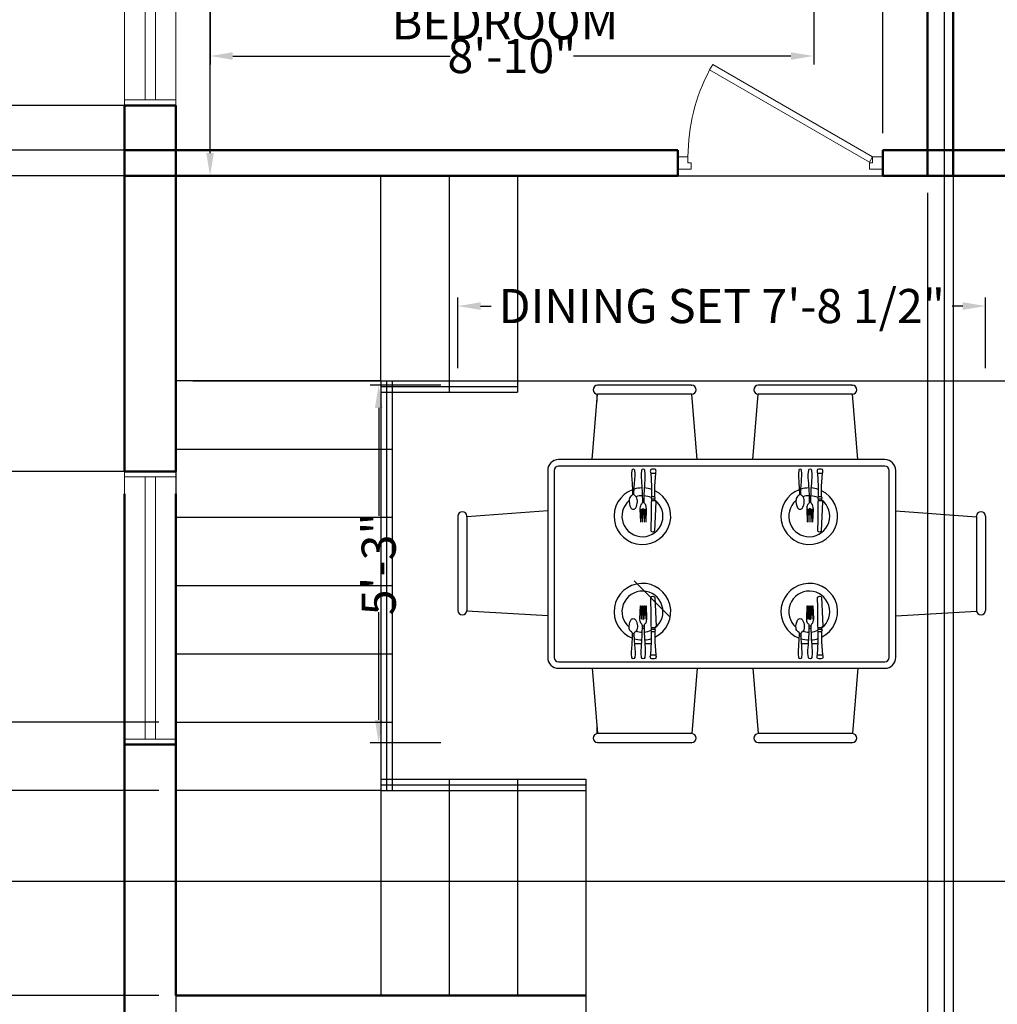
# Model space of a CAD drawing. Units: inches. Extents: x 6704 to 7574, y 11759 to 12617.
# Tile 4 of 8: x 6900 to 7071, y 12195 to 12368. Entities that reach past the tile are written whole.
import ezdxf

# ---------------------------------------------------------------- set-up
doc = ezdxf.new("R2010")
doc.units = ezdxf.units.IN
doc.header["$MEASUREMENT"] = 0
doc.layers.add('a patt', color=33, linetype='Continuous')
for name, color, linetype, lineweight in [('A-AREA-IDEN', 7, 'Continuous', 18), ('A-DOOR', 4, 'Continuous', 20), ('A-FLOR-STRS', 7, 'Continuous', 25), ('A-FURN', 8, 'Continuous', 18), ('WALL', 7, 'Continuous', 50), ('WINDOW', 2, 'Continuous', 20), ('YQ_DIM', 3, 'Continuous', 18)]:
    doc.layers.add(name, color=color, linetype=linetype, lineweight=lineweight)
doc.styles.get("Standard").update_dxf_attribs({"font": 'arial.ttf'})
doc.styles.add('YQ_DIM', font='SUPEROS.SHX', dxfattribs={"width": 0.8, "bigfont": 'HZDX.SHX'})
doc.dimstyles.new('yqi0', dxfattribs={"dimscale": 0, "dimtxt": 6, "dimasz": 4, "dimexe": 1.5, "dimexo": 3, "dimgap": 0.5, "dimtad": 0, "dimdsep": 46, "dimlunit": 4, "dimtxsty": 'Standard', "dimcen": 0, "dimclrd": 256, "dimclre": 256, "dimclrt": 7, "dimadec": 1, "dimazin": 2, "dimtfac": 1, "dimtix": 1, "dimtmove": 2, "dimatfit": 2, "dimfxl": 1, "dimtolj": 1, "dimtzin": 0, "dimarcsym": 0})

# ---------------------------------------------------------------- blocks, each defined once
blk = doc.blocks.new('*D4')
at = {"layer": 'Defpoints', "color": 0, "transparency": 16777216}
for p in [(6927.07, 12502.26), (6927.07, 12340.26), (6933.07, 12340.26)]:
    blk.add_point(p, dxfattribs=at)
at = {"layer": 'YQ_DIM', "color": 0, "lineweight": -2, "transparency": 16777216}
for p, q in [((6930.07, 12502.26), (6934.57, 12502.26)), ((6933.07, 12498.26), (6933.07, 12431.78)), ((6933.07, 12344.26), (6933.07, 12410.73)), ((6930.07, 12340.26), (6934.57, 12340.26))]:
    blk.add_line(p, q, dxfattribs=at)
at = {"layer": 'YQ_DIM', "color": 0, "transparency": 16777216}
for points in [[(6932.41, 12498.26), (6933.74, 12498.26), (6933.07, 12502.26)], [(6932.41, 12344.26), (6933.74, 12344.26), (6933.07, 12340.26)]]:
    blk.add_solid(points, dxfattribs=at)
at = {"layer": 'YQ_DIM', "color": 0, "transparency": 16777216, "insert": (6933.07, 12421.26), "char_height": 6, "attachment_point": 5, "rotation": 90}
blk.add_mtext('\\A1;13\'-6"', dxfattribs=at)
blk = doc.blocks.new('WD_00_X1')
for p, q in [((-0.5, 0.5), (0.5, 0.5)), ((-0.48, 0.5), (-0.48, -0.5)), ((0.48, 0.5), (0.48, -0.5)), ((0.48, 0.1), (-0.48, 0.1)), ((0.48, -0.1), (-0.48, -0.1)), ((-0.5, -0.5), (0.5, -0.5))]:
    blk.add_line(p, q)
blk = doc.blocks.new('DR_CDR1')
for p, q in [((0.3294, 0.48), (-0.45, 0.03)), ((-0.435, 0.004), (0.3444, 0.454)), ((0.3294, 0.48), (0.3444, 0.454)), ((-0.45, 0.03), (-0.5, 0.03)), ((-0.435, 0.004), (-0.45, 0.03)), ((-0.45, 0.03), (-0.45, 0)), ((-0.45, 0), (-0.435, 0)), ((-0.435, 0), (-0.435, -0.03)), ((0.435, 0), (0.45, 0)), ((0.435, 0), (0.435, -0.03)), ((0.45, 0.03), (0.45, 0)), ((0.5, 0.03), (0.45, 0.03)), ((-0.435, -0.03), (-0.5, -0.03)), ((0.435, -0.03), (0.5, -0.03))]:
    blk.add_line(p, q)
blk.add_lwpolyline([(0.3444, 0.454, -0.121959), (0.45, 0.03)], format="xyb")
blk = doc.blocks.new('grdfg')
at = {"layer": 'a patt'}
for p, q in [((615.1, 1349.1), (612, 1348.9)), ((1015.8, 1349), (615, 1349)), ((615, 1348.9), (615, 1349)), ((1015.8, 1349.1), (1018.9, 1348.9)), ((1307.5, 1349.1), (1304.3, 1348.9)), ((1307.4, 1348.9), (1307.4, 1349)), ((1708.1, 1349), (1307.4, 1349)), ((1708.1, 1349.1), (1711.2, 1348.9)), ((589, 1028.2), (611.9, 1309.9)), ((609.3, 1310.2), (609.3, 1278.3)), ((1018.9, 1309.9), (611.8, 1309.9)), ((1041.8, 1028.2), (1018.9, 1310)), ((1281.4, 1028.2), (1304.2, 1309.9)), ((1711.2, 1309.9), (1304.2, 1309.9)), ((1734.1, 1028.2), (1711.3, 1310)), ((605.1, 1201.3), (603.1, 1201.3)), ((1297.4, 1201.3), (1295.4, 1201.3)), ((1850.7, 1028.2), (443.9, 1028.2)), ((397.3, 981.6), (397.3, 174.8)), ((425.3, 981.6), (425.3, 174.8)), ((1850.7, 1000.2), (443.9, 1000.2)), ((1869.3, 174.8), (1869.3, 981.6)), ((1897.3, 174.8), (1897.3, 981.6)), ((841.2, 969.6), (862.7, 969.6)), ((1560.1, 969.6), (1581.7, 969.6)), ((763.3, 888.1), (769.2, 888.1)), ((763.3, 878.9), (769.2, 878.9)), ((812.6, 857.1), (805.6, 857.1)), ((844.8, 869.7), (859.1, 869.7)), ((844.8, 858.9), (859.1, 858.9)), ((844.8, 851.7), (859.1, 851.7)), ((1482.3, 888.1), (1488.2, 888.1)), ((1482.3, 878.9), (1488.2, 878.9)), ((1531.6, 857.1), (1524.6, 857.1)), ((1563.7, 869.7), (1578.1, 869.7)), ((1563.7, 858.9), (1578.1, 858.9)), ((1563.7, 851.7), (1578.1, 851.7)), ((397.3, 807.5), (49.1, 781.7)), ((805.6, 844.8), (812.6, 844.8)), ((1524.6, 844.8), (1531.6, 844.8)), ((1897.3, 807.5), (2245.5, 781.7)), ((10, 784.9), (10, 377.8)), ((49.2, 781.8), (49, 784.9)), ((49.1, 781.7), (49.1, 381)), ((2245.4, 781.8), (2245.6, 784.9)), ((2245.5, 781.7), (2245.5, 381)), ((2284.6, 784.9), (2284.6, 377.8)), ((769.7, 504.8), (923, 351.5)), ((397.3, 355.1), (48.7, 375)), ((49.2, 381.1), (49, 378)), ((49, 381), (49.1, 381)), ((1897.3, 355.1), (2245.9, 375)), ((2245.4, 381.1), (2245.6, 378)), ((2245.6, 381), (2245.5, 381)), ((805.6, 311.6), (812.6, 311.6)), ((812.6, 299.3), (805.6, 299.3)), ((844.8, 304.7), (859.1, 304.7)), ((844.8, 297.5), (859.1, 297.5)), ((1524.6, 311.6), (1531.6, 311.6)), ((1531.6, 299.3), (1524.6, 299.3)), ((1563.7, 304.7), (1578.1, 304.7)), ((1563.7, 297.5), (1578.1, 297.5)), ((763.3, 277.5), (769.2, 277.5)), ((763.3, 268.3), (769.2, 268.3)), ((844.8, 286.7), (859.1, 286.7)), ((1482.3, 277.5), (1488.2, 277.5)), ((1482.3, 268.3), (1488.2, 268.3)), ((1563.7, 286.7), (1578.1, 286.7)), ((771, 235), (802.4, 235)), ((815.8, 235), (844.3, 235)), ((1490, 235), (1521.4, 235)), ((1534.8, 235), (1563.3, 235)), ((841.2, 186.8), (862.7, 186.8)), ((1560.1, 186.8), (1581.7, 186.8)), ((443.9, 156.2), (1850.7, 156.2)), ((443.9, 128.2), (1850.7, 128.2)), ((589, 128.2), (611.9, -153.5)), ((1041.8, 128.2), (1018.9, -153.6)), ((1281.4, 128.2), (1304.2, -153.5)), ((1734.1, 128.2), (1711.3, -153.6)), ((605.1, -44.9), (603.1, -44.9)), ((1027.7, -44.9), (1025.6, -44.9)), ((609.3, -122), (609.3, -153.8)), ((1018.9, -153.5), (611.8, -153.5)), ((1711.2, -153.5), (1304.2, -153.5)), ((615.1, -192.7), (612, -192.5)), ((615, -192.5), (615, -192.6)), ((1015.8, -192.6), (615, -192.6)), ((1015.8, -192.7), (1018.9, -192.5)), ((1307.5, -192.7), (1304.3, -192.5)), ((1307.4, -192.5), (1307.4, -192.6)), ((1708.1, -192.6), (1307.4, -192.6)), ((1708.1, -192.7), (1711.2, -192.5))]:
    blk.add_line(p, q, dxfattribs=at)
for points in [[(758.7, 967), (758.7, 954.7, -0.013852), (763.3, 888.1), (763.3, 878.9, -0.321801), (757.9, 871.5, 0.220637), (748.8, 856.4, 0.151079), (755.6, 820.3, 0.601255), (776.8, 820.3, 0.098298), (784.5, 845.7, 0.173345), (779.1, 866.9, 0.127575), (772.3, 873, -0.108886), (769.2, 878.9), (769.2, 888.1, -0.013852), (773.8, 954.7), (773.8, 967), (772.3, 982, 0.903848), (760.2, 982)], [(841.2, 985.7, 0.204141), (841.2, 969.6), (844.8, 914.2), (844.8, 869.7), (843, 862.5), (844.8, 858.9), (844.8, 851.7), (843, 846.6, -0.015744), (841.2, 721.5, 0.538165), (859.1, 721.5), (864.3, 846.6), (859.1, 851.7), (859.1, 858.9), (860.9, 862.5), (859.1, 869.7), (859.1, 914.2), (862.7, 969.6, 0.204141), (862.7, 985.7), (857.3, 987.5), (846.6, 987.5)], [(1477.7, 967), (1477.7, 954.7, -0.013852), (1482.3, 888.1), (1482.3, 878.9, -0.321801), (1476.9, 871.5, 0.220637), (1467.8, 856.4, 0.151079), (1474.6, 820.3, 0.601255), (1495.8, 820.3, 0.098298), (1503.5, 845.7, 0.173345), (1498.1, 866.9, 0.127575), (1491.2, 873, -0.108886), (1488.2, 878.9), (1488.2, 888.1, -0.013852), (1492.8, 954.7), (1492.8, 967), (1491.2, 982, 0.903848), (1479.2, 982)], [(1560.1, 985.7, 0.204141), (1560.1, 969.6), (1563.7, 914.2), (1563.7, 869.7), (1561.9, 862.5), (1563.7, 858.9), (1563.7, 851.7), (1561.9, 846.6, -0.015744), (1560.1, 721.5, 0.538165), (1578.1, 721.5), (1583.3, 846.6), (1578.1, 851.7), (1578.1, 858.9), (1579.9, 862.5), (1578.1, 869.7), (1578.1, 914.2), (1581.7, 969.6, 0.204141), (1581.7, 985.7), (1576.3, 987.5), (1565.5, 987.5)], [(841.2, 170.6, -0.204141), (841.2, 186.8), (844.8, 242.1), (844.8, 286.7), (843, 293.9), (844.8, 297.5), (844.8, 304.7), (843, 309.8, 0.015744), (841.2, 434.9, -0.538165), (859.1, 434.9), (864.3, 309.8), (859.1, 304.7), (859.1, 297.5), (860.9, 293.9), (859.1, 286.7), (859.1, 242.1), (862.7, 186.8, -0.204141), (862.7, 170.6), (857.3, 168.8), (846.6, 168.8)], [(1560.1, 170.6, -0.204141), (1560.1, 186.8), (1563.7, 242.1), (1563.7, 286.7), (1561.9, 293.9), (1563.7, 297.5), (1563.7, 304.7), (1561.9, 309.8, 0.015744), (1560.1, 434.9, -0.538165), (1578.1, 434.9), (1583.3, 309.8), (1578.1, 304.7), (1578.1, 297.5), (1579.9, 293.9), (1578.1, 286.7), (1578.1, 242.1), (1581.7, 186.8, -0.204141), (1581.7, 170.6), (1576.3, 168.8), (1565.5, 168.8)], [(758.7, 189.4), (758.7, 201.7, 0.013852), (763.3, 268.3), (763.3, 277.5, 0.321801), (757.9, 284.9, -0.220637), (748.8, 300, -0.151079), (755.6, 336.1, -0.601255), (776.8, 336.1, -0.098298), (784.5, 310.7, -0.173345), (779.1, 289.5, -0.127575), (772.3, 283.4, 0.108886), (769.2, 277.5), (769.2, 268.3, 0.013852), (773.8, 201.7), (773.8, 189.4), (772.3, 174.3, -0.903848), (760.2, 174.3)], [(1477.7, 189.4), (1477.7, 201.7, 0.013852), (1482.3, 268.3), (1482.3, 277.5, 0.321801), (1476.9, 284.9, -0.220637), (1467.8, 300, -0.151079), (1474.6, 336.1, -0.601255), (1495.8, 336.1, -0.098298), (1503.5, 310.7, -0.173345), (1498.1, 289.5, -0.127575), (1491.2, 283.4, 0.108886), (1488.2, 277.5), (1488.2, 268.3, 0.013852), (1492.8, 201.7), (1492.8, 189.4), (1491.2, 174.3, -0.903848), (1479.2, 174.3)]]:
    blk.add_lwpolyline(points, format="xyb", close=True, dxfattribs=at)
for points in [[(802, 981.9), (800.2, 964.2), (800.2, 950, -0.012883), (805.6, 857.1), (805.6, 844.8, -0.236068), (798.4, 834, 0.098033), (794.8, 814.4), (796.6, 759.1), (798.4, 759.1), (800.2, 814.4), (802, 814.4), (803.8, 759.1), (805.6, 759.1), (807.4, 816.2), (809.2, 818), (810.8, 816.2), (812.6, 759.1), (814.4, 759.1), (816.2, 814.4), (818, 814.4), (819.8, 759.1), (821.6, 759.1), (823.4, 814.4), (819.8, 834, -0.236068), (812.6, 844.8), (812.6, 857.1, -0.012883), (818, 950), (818, 964.2), (816.2, 981.9, 0.761905), (802, 981.9, 0.027392)], [(1521, 981.9), (1519.2, 964.2), (1519.2, 950, -0.012883), (1524.6, 857.1), (1524.6, 844.8, -0.236068), (1517.4, 834, 0.098033), (1513.8, 814.4), (1515.6, 759.1), (1517.4, 759.1), (1519.2, 814.4), (1521, 814.4), (1522.8, 759.1), (1524.6, 759.1), (1526.4, 816.2), (1528.2, 818), (1529.8, 816.2), (1531.6, 759.1), (1533.4, 759.1), (1535.2, 814.4), (1537, 814.4), (1538.8, 759.1), (1540.6, 759.1), (1542.4, 814.4), (1538.8, 834, -0.236068), (1531.6, 844.8), (1531.6, 857.1, -0.012883), (1537, 950), (1537, 964.2), (1535.2, 981.9, 0.761905), (1521, 981.9, 0.027392)], [(802, 174.5), (800.2, 192.2), (800.2, 206.4, 0.012883), (805.6, 299.3), (805.6, 311.6, 0.236068), (798.4, 322.4, -0.098033), (794.8, 342), (796.6, 397.3), (798.4, 397.3), (800.2, 342), (802, 342), (803.8, 397.3), (805.6, 397.3), (807.4, 340.2), (809.2, 338.4), (810.8, 340.2), (812.6, 397.3), (814.4, 397.3), (816.2, 342), (818, 342), (819.8, 397.3), (821.6, 397.3), (823.4, 342), (819.8, 322.4, 0.236068), (812.6, 311.6), (812.6, 299.3, 0.012883), (818, 206.4), (818, 192.2), (816.2, 174.5, -0.761905), (802, 174.5, -0.027392)], [(1521, 174.5), (1519.2, 192.2), (1519.2, 206.4, 0.012883), (1524.6, 299.3), (1524.6, 311.6, 0.236068), (1517.4, 322.4, -0.098033), (1513.8, 342), (1515.6, 397.3), (1517.4, 397.3), (1519.2, 342), (1521, 342), (1522.8, 397.3), (1524.6, 397.3), (1526.4, 340.2), (1528.2, 338.4), (1529.8, 340.2), (1531.6, 397.3), (1533.4, 397.3), (1535.2, 342), (1537, 342), (1538.8, 397.3), (1540.6, 397.3), (1542.4, 342), (1538.8, 322.4, 0.236068), (1531.6, 311.6), (1531.6, 299.3, 0.012883), (1537, 206.4), (1537, 192.2), (1535.2, 174.5, -0.761905), (1521, 174.5, -0.027392)]]:
    blk.add_lwpolyline(points, format="xyb", dxfattribs=at)
for centre, radius, start, end in [((612.9, 1329.4), 19.5, 92.4912, 267.9051), ((1018, 1329.4), 19.5, 272.0949, 87.5088), ((1305.2, 1329.4), 19.5, 92.4912, 267.9051), ((1710.4, 1329.4), 19.5, 272.0949, 87.5088), ((443.9, 981.6), 46.6, 90, 180), ((1850.7, 981.6), 46.6, 0, 90), ((443.9, 981.6), 18.7, 90, 180), ((1850.7, 981.6), 18.7, 0, 90), ((805.7, 784), 122.1, 110.569, 64.0676), ((805.7, 784), 122.1, 91.1026, 107.1168), ((805.7, 784), 122.1, 71.3681, 85.7295), ((1524.7, 784), 122.1, 110.569, 64.0676), ((1524.7, 784), 122.1, 91.1026, 107.1168), ((1524.7, 784), 122.1, 71.3681, 85.7295), ((805.7, 784), 88.4, 130.4177, 52.8326), ((805.7, 784), 88.4, 90.4281, 108.0635), ((805.7, 784), 88.4, 64.8376, 85.191), ((1524.7, 784), 88.4, 130.4177, 52.8326), ((1524.7, 784), 88.4, 90.4281, 108.0635), ((1524.7, 784), 88.4, 64.8376, 85.191), ((29.5, 784), 19.5, 2.4912, 177.9051), ((2265.1, 784), 19.5, 2.0949, 177.5088), ((805.7, 372.4), 122.1, 295.9324, 249.431), ((1524.7, 372.4), 122.1, 295.9324, 249.431), ((805.7, 372.4), 88.4, 307.1674, 229.5823), ((1524.7, 372.4), 88.4, 307.1674, 229.5823), ((29.5, 378.8), 19.5, 182.0949, 357.5088), ((2265.1, 378.8), 19.5, 182.4912, 357.9051), ((805.7, 372.4), 122.1, 252.8832, 268.8974), ((805.7, 372.4), 88.4, 251.9365, 269.5719), ((805.7, 372.4), 88.4, 274.809, 295.1624), ((805.7, 372.4), 122.1, 274.2705, 288.6319), ((1524.7, 372.4), 122.1, 252.8832, 268.8974), ((1524.7, 372.4), 88.4, 251.9365, 269.5719), ((1524.7, 372.4), 88.4, 274.809, 295.1624), ((1524.7, 372.4), 122.1, 274.2705, 288.6319), ((443.9, 174.8), 46.6, 180, 270), ((443.9, 174.8), 18.7, 180, 270), ((1850.7, 174.8), 46.6, 270, 0), ((1850.7, 174.8), 18.7, 270, 0), ((612.9, -173), 19.5, 92.0949, 267.5088), ((1018, -173), 19.5, 272.4912, 87.9051), ((1305.2, -173), 19.5, 92.0949, 267.5088), ((1710.4, -173), 19.5, 272.4912, 87.9051)]:
    blk.add_arc(centre, radius, start, end, dxfattribs=at)
blk = doc.blocks.new('*D40')
at = {"layer": 'Defpoints', "color": 0, "transparency": 16777216}
for p in [(6933.07, 12377.5), (7039.07, 12377.5), (6933.07, 12361.3)]:
    blk.add_point(p, dxfattribs=at)
at = {"layer": 'YQ_DIM', "lineweight": -2, "transparency": 16777216}
for p, q in [((6933.07, 12374.5), (6933.07, 12359.8)), ((7039.07, 12374.5), (7039.07, 12359.8)), ((6937.07, 12361.3), (6975.26, 12361.3)), ((7035.07, 12361.3), (6996.88, 12361.3))]:
    blk.add_line(p, q, dxfattribs=at)
at = {"layer": 'YQ_DIM', "transparency": 16777216}
for points in [[(6937.07, 12361.96), (6937.07, 12360.63), (6933.07, 12361.3)], [(7035.07, 12361.96), (7035.07, 12360.63), (7039.07, 12361.3)]]:
    blk.add_solid(points, dxfattribs=at)
at = {"layer": 'YQ_DIM', "color": 7, "transparency": 16777216, "insert": (6986.07, 12361.3), "char_height": 6, "attachment_point": 5}
blk.add_mtext('\\A1;8\'-10"', dxfattribs=at)
blk = doc.blocks.new('*D45')
at = {"layer": 'Defpoints', "color": 0, "transparency": 16777216}
for p in [(7069.25, 12317.37), (6976.59, 12303.47), (7069.25, 12303.47)]:
    blk.add_point(p, dxfattribs=at)
at = {"layer": 'YQ_DIM', "lineweight": -2, "transparency": 16777216}
for p, q in [((6976.59, 12306.47), (6976.59, 12318.87)), ((7069.25, 12306.47), (7069.25, 12318.87)), ((6980.59, 12317.37), (6982.45, 12317.37)), ((7065.25, 12317.37), (7063.38, 12317.37))]:
    blk.add_line(p, q, dxfattribs=at)
at = {"layer": 'YQ_DIM', "transparency": 16777216}
for points in [[(6980.59, 12318.04), (6980.59, 12316.7), (6976.59, 12317.37)], [(7065.25, 12318.04), (7065.25, 12316.7), (7069.25, 12317.37)]]:
    blk.add_solid(points, dxfattribs=at)
at = {"layer": 'YQ_DIM', "color": 7, "transparency": 16777216, "insert": (7022.92, 12317.37), "char_height": 6, "attachment_point": 5}
blk.add_mtext('\\A1;DINING SET 7\'-8 1/2"', dxfattribs=at)
blk = doc.blocks.new('*D46')
at = {"layer": 'Defpoints', "color": 0, "transparency": 16777216}
for p in [(6962.69, 12303.47), (6976.59, 12303.47), (6976.59, 12240.67)]:
    blk.add_point(p, dxfattribs=at)
at = {"layer": 'YQ_DIM', "lineweight": -2, "transparency": 16777216}
for p, q in [((6973.59, 12303.47), (6961.19, 12303.47)), ((6962.69, 12299.47), (6962.69, 12280.54)), ((6962.69, 12244.67), (6962.69, 12263.59)), ((6973.59, 12240.67), (6961.19, 12240.67))]:
    blk.add_line(p, q, dxfattribs=at)
at = {"layer": 'YQ_DIM', "transparency": 16777216}
for points in [[(6962.02, 12299.47), (6963.36, 12299.47), (6962.69, 12303.47)], [(6962.02, 12244.67), (6963.36, 12244.67), (6962.69, 12240.67)]]:
    blk.add_solid(points, dxfattribs=at)
at = {"layer": 'YQ_DIM', "color": 7, "transparency": 16777216, "insert": (6962.69, 12272.07), "char_height": 6, "attachment_point": 5, "rotation": 90}
blk.add_mtext('\\A1;5\'-3"', dxfattribs=at)
blk = doc.blocks.new('*D56')
at = {"layer": 'Defpoints', "color": 0, "transparency": 16777216}
for p in [(6712.97, 12511.26), (6918.07, 12511.26), (6918.07, 12011.76)]:
    blk.add_point(p, dxfattribs=at)
at = {"layer": 'YQ_DIM', "lineweight": -2, "transparency": 16777216}
for p, q in [((6915.07, 12511.26), (6711.47, 12511.26)), ((6712.97, 12507.26), (6712.97, 12279.42)), ((6712.97, 12015.76), (6712.97, 12243.59)), ((6915.07, 12011.76), (6711.47, 12011.76))]:
    blk.add_line(p, q, dxfattribs=at)
at = {"layer": 'YQ_DIM', "transparency": 16777216}
for points in [[(6712.3, 12507.26), (6713.64, 12507.26), (6712.97, 12511.26)], [(6712.3, 12015.76), (6713.64, 12015.76), (6712.97, 12011.76)]]:
    blk.add_solid(points, dxfattribs=at)
at = {"layer": 'YQ_DIM', "color": 7, "transparency": 16777216, "insert": (6712.97, 12261.51), "char_height": 6, "attachment_point": 5, "rotation": 90}
blk.add_mtext('\\A1;41\'-7 1/2"', dxfattribs=at)
blk = doc.blocks.new('*D59')
at = {"layer": 'Defpoints', "color": 0, "transparency": 16777216}
for p in [(6927.07, 12344.76), (7059.07, 12340.26), (7059.07, 11768.08)]:
    blk.add_point(p, dxfattribs=at)
at = {"layer": 'YQ_DIM', "lineweight": -2, "transparency": 16777216}
for p, q in [((6927.07, 12341.76), (6927.07, 11766.58)), ((7059.07, 12337.26), (7059.07, 11766.58)), ((6931.07, 11768.08), (6982.55, 11768.08)), ((7055.07, 11768.08), (7003.6, 11768.08))]:
    blk.add_line(p, q, dxfattribs=at)
at = {"layer": 'YQ_DIM', "transparency": 16777216}
for points in [[(6931.07, 11768.74), (6931.07, 11767.41), (6927.07, 11768.08)], [(7055.07, 11768.74), (7055.07, 11767.41), (7059.07, 11768.08)]]:
    blk.add_solid(points, dxfattribs=at)
at = {"layer": 'YQ_DIM', "color": 7, "transparency": 16777216, "insert": (6993.07, 11768.08), "char_height": 6, "attachment_point": 5}
blk.add_mtext('\\A1;11\'-0"', dxfattribs=at)
blk = doc.blocks.new('*D60')
at = {"layer": 'Defpoints', "color": 0, "transparency": 16777216}
for p in [(7063.57, 12400.26), (7117.57, 12400.26), (7117.57, 11768.08)]:
    blk.add_point(p, dxfattribs=at)
at = {"layer": 'YQ_DIM', "lineweight": -2, "transparency": 16777216}
for p, q in [((7063.57, 12397.26), (7063.57, 11766.58)), ((7117.57, 12397.26), (7117.57, 11766.58)), ((7067.57, 11768.08), (7081.98, 11768.08)), ((7113.57, 11768.08), (7099.17, 11768.08))]:
    blk.add_line(p, q, dxfattribs=at)
at = {"layer": 'YQ_DIM', "transparency": 16777216}
for points in [[(7067.57, 11768.74), (7067.57, 11767.41), (7063.57, 11768.08)], [(7113.57, 11768.74), (7113.57, 11767.41), (7117.57, 11768.08)]]:
    blk.add_solid(points, dxfattribs=at)
at = {"layer": 'YQ_DIM', "color": 7, "transparency": 16777216, "insert": (7090.57, 11768.08), "char_height": 6, "attachment_point": 5}
blk.add_mtext('\\A1;4\'-6"', dxfattribs=at)
blk = doc.blocks.new('*D65')
at = {"layer": 'Defpoints', "color": 0, "transparency": 16777216}
for p in [(7113.07, 12590.81), (7062.07, 12121.26), (7113.07, 12121.26)]:
    blk.add_point(p, dxfattribs=at)
at = {"layer": 'YQ_DIM', "lineweight": -2, "transparency": 16777216}
for p, q in [((7062.07, 12124.26), (7062.07, 12592.31)), ((7113.07, 12124.26), (7113.07, 12592.31)), ((7066.07, 12590.81), (7078.98, 12590.81)), ((7109.07, 12590.81), (7096.17, 12590.81))]:
    blk.add_line(p, q, dxfattribs=at)
at = {"layer": 'YQ_DIM', "transparency": 16777216}
for points in [[(7066.07, 12591.47), (7066.07, 12590.14), (7062.07, 12590.81)], [(7109.07, 12591.47), (7109.07, 12590.14), (7113.07, 12590.81)]]:
    blk.add_solid(points, dxfattribs=at)
at = {"layer": 'YQ_DIM', "color": 7, "transparency": 16777216, "insert": (7087.57, 12590.81), "char_height": 6, "attachment_point": 5}
blk.add_mtext('\\A1;4\'-3"', dxfattribs=at)
blk = doc.blocks.new('*D67')
at = {"layer": 'Defpoints', "color": 0, "transparency": 16777216}
for p in [(6712.97, 12340.26), (6927.07, 12340.26), (6927.07, 12196.26)]:
    blk.add_point(p, dxfattribs=at)
at = {"layer": 'YQ_DIM', "lineweight": -2, "transparency": 16777216}
for p, q in [((6924.07, 12340.26), (6711.47, 12340.26)), ((6712.97, 12336.26), (6712.97, 12278.78)), ((6712.97, 12200.26), (6712.97, 12257.73)), ((6924.07, 12196.26), (6711.47, 12196.26))]:
    blk.add_line(p, q, dxfattribs=at)
at = {"layer": 'YQ_DIM', "transparency": 16777216}
for points in [[(6712.3, 12336.26), (6713.64, 12336.26), (6712.97, 12340.26)], [(6712.3, 12200.26), (6713.64, 12200.26), (6712.97, 12196.26)]]:
    blk.add_solid(points, dxfattribs=at)
at = {"layer": 'YQ_DIM', "color": 7, "transparency": 16777216, "insert": (6712.97, 12268.26), "char_height": 6, "attachment_point": 5, "rotation": 90}
blk.add_mtext('\\A1;12\'-0"', dxfattribs=at)
blk = doc.blocks.new('*D68')
at = {"layer": 'Defpoints', "color": 0, "transparency": 16777216}
for p in [(6927.07, 12340.26), (7565.25, 12340.26), (6927.07, 12304.26)]:
    blk.add_point(p, dxfattribs=at)
at = {"layer": 'YQ_DIM', "lineweight": -2, "transparency": 16777216}
for p, q in [((6930.07, 12340.26), (7566.75, 12340.26)), ((7565.25, 12336.26), (7565.25, 12330.73)), ((7565.25, 12308.26), (7565.25, 12313.78)), ((6930.07, 12304.26), (7566.75, 12304.26))]:
    blk.add_line(p, q, dxfattribs=at)
at = {"layer": 'YQ_DIM', "transparency": 16777216}
for points in [[(7564.58, 12336.26), (7565.91, 12336.26), (7565.25, 12340.26)], [(7564.58, 12308.26), (7565.91, 12308.26), (7565.25, 12304.26)]]:
    blk.add_solid(points, dxfattribs=at)
at = {"layer": 'YQ_DIM', "color": 7, "transparency": 16777216, "insert": (7565.25, 12322.26), "char_height": 6, "attachment_point": 5, "rotation": 90}
blk.add_mtext('\\A1;3\'-0"', dxfattribs=at)
blk = doc.blocks.new('*D77')
at = {"layer": 'Defpoints', "color": 0, "transparency": 16777216}
for p in [(7260.07, 12216.3), (6712.97, 12173.76), (7260.07, 12173.76)]:
    blk.add_point(p, dxfattribs=at)
at = {"layer": 'YQ_DIM', "lineweight": -2, "transparency": 16777216}
for p, q in [((7257.07, 12216.3), (6711.47, 12216.3)), ((6712.97, 12212.3), (6712.97, 12210.49)), ((6712.97, 12177.76), (6712.97, 12179.57)), ((7257.07, 12173.76), (6711.47, 12173.76))]:
    blk.add_line(p, q, dxfattribs=at)
at = {"layer": 'YQ_DIM', "transparency": 16777216}
for points in [[(6712.3, 12212.3), (6713.64, 12212.3), (6712.97, 12216.3)], [(6712.3, 12177.76), (6713.64, 12177.76), (6712.97, 12173.76)]]:
    blk.add_solid(points, dxfattribs=at)
at = {"layer": 'YQ_DIM', "color": 7, "transparency": 16777216, "insert": (6712.97, 12195.03), "char_height": 6, "attachment_point": 5, "rotation": 90}
blk.add_mtext('\\A1;3\'-6 1/2"', dxfattribs=at)
blk = doc.blocks.new('*D78')
at = {"layer": 'Defpoints', "color": 0, "transparency": 16777216}
for p in [(6712.97, 12352.63), (6927.07, 12352.63), (6927.07, 12344.76)]:
    blk.add_point(p, dxfattribs=at)
at = {"layer": 'YQ_DIM', "lineweight": -2, "transparency": 16777216}
for p, q in [((6712.97, 12356.63), (6712.97, 12360.63)), ((6924.07, 12352.63), (6711.47, 12352.63)), ((6712.97, 12344.76), (6712.97, 12352.63)), ((6924.07, 12344.76), (6711.47, 12344.76)), ((6712.97, 12340.76), (6712.97, 12336.76))]:
    blk.add_line(p, q, dxfattribs=at)
at = {"layer": 'YQ_DIM', "transparency": 16777216}
for points in [[(6712.3, 12356.63), (6713.64, 12356.63), (6712.97, 12352.63)], [(6712.3, 12340.76), (6713.64, 12340.76), (6712.97, 12344.76)]]:
    blk.add_solid(points, dxfattribs=at)
at = {"layer": 'YQ_DIM', "color": 7, "transparency": 16777216, "insert": (6712.97, 12348.69), "char_height": 6, "attachment_point": 5, "rotation": 90}
blk.add_mtext('\\A1;0\'-8"', dxfattribs=at)
blk = doc.blocks.new('*D83')
at = {"layer": 'Defpoints', "color": 0, "transparency": 16777216}
for p in [(7051.2, 12590.81), (7051.2, 12344.76), (7059.07, 12340.26)]:
    blk.add_point(p, dxfattribs=at)
at = {"layer": 'YQ_DIM', "lineweight": -2, "transparency": 16777216}
for p, q in [((7051.2, 12347.76), (7051.2, 12592.31)), ((7059.07, 12343.26), (7059.07, 12592.31)), ((7047.2, 12590.81), (7043.2, 12590.81)), ((7059.07, 12590.81), (7051.2, 12590.81)), ((7063.07, 12590.81), (7067.07, 12590.81))]:
    blk.add_line(p, q, dxfattribs=at)
at = {"layer": 'YQ_DIM', "transparency": 16777216}
for points in [[(7047.2, 12591.47), (7047.2, 12590.14), (7051.2, 12590.81)], [(7063.07, 12591.47), (7063.07, 12590.14), (7059.07, 12590.81)]]:
    blk.add_solid(points, dxfattribs=at)
at = {"layer": 'YQ_DIM', "color": 7, "transparency": 16777216, "insert": (7055.14, 12590.81), "char_height": 6, "attachment_point": 5}
blk.add_mtext('\\A1;0\'-8"', dxfattribs=at)
blk = doc.blocks.new('*D86')
at = {"layer": 'Defpoints', "color": 0, "transparency": 16777216}
for p in [(6712.97, 12340.26), (6927.07, 12340.26), (6927.07, 12288.32)]:
    blk.add_point(p, dxfattribs=at)
at = {"layer": 'YQ_DIM', "lineweight": -2, "transparency": 16777216}
for p, q in [((6924.07, 12340.26), (6711.47, 12340.26)), ((6712.97, 12336.26), (6712.97, 12322.88)), ((6712.97, 12292.32), (6712.97, 12305.69)), ((6924.07, 12288.32), (6711.47, 12288.32))]:
    blk.add_line(p, q, dxfattribs=at)
at = {"layer": 'YQ_DIM', "transparency": 16777216}
for points in [[(6712.3, 12336.26), (6713.64, 12336.26), (6712.97, 12340.26)], [(6712.3, 12292.32), (6713.64, 12292.32), (6712.97, 12288.32)]]:
    blk.add_solid(points, dxfattribs=at)
at = {"layer": 'YQ_DIM', "color": 7, "transparency": 16777216, "insert": (6712.97, 12314.29), "char_height": 6, "attachment_point": 5, "rotation": 90}
blk.add_mtext('\\A1;4\'-4"', dxfattribs=at)
blk = doc.blocks.new('*D87')
at = {"layer": 'Defpoints', "color": 0, "transparency": 16777216}
for p in [(6712.97, 12244.26), (6927.07, 12244.26), (6927.07, 12232.26)]:
    blk.add_point(p, dxfattribs=at)
at = {"layer": 'YQ_DIM', "lineweight": -2, "transparency": 16777216}
for p, q in [((6712.97, 12248.26), (6712.97, 12252.26)), ((6924.07, 12244.26), (6711.47, 12244.26)), ((6712.97, 12232.26), (6712.97, 12244.26)), ((6924.07, 12232.26), (6711.47, 12232.26)), ((6712.97, 12228.26), (6712.97, 12224.26))]:
    blk.add_line(p, q, dxfattribs=at)
at = {"layer": 'YQ_DIM', "transparency": 16777216}
for points in [[(6712.3, 12248.26), (6713.64, 12248.26), (6712.97, 12244.26)], [(6712.3, 12228.26), (6713.64, 12228.26), (6712.97, 12232.26)]]:
    blk.add_solid(points, dxfattribs=at)
at = {"layer": 'YQ_DIM', "color": 7, "transparency": 16777216, "insert": (6712.97, 12238.26), "char_height": 6, "attachment_point": 5, "rotation": 90}
blk.add_mtext('\\A1;1\'-0"', dxfattribs=at)

msp = doc.modelspace()

# ---------------------------------------------------------------- linework, layer by layer
at = {"layer": 'A-FLOR-STRS'}
for p, q in [((6963.073, 12304.257), (6963.073, 12340.257)), ((6975.073, 12340.257), (6975.073, 12302.257)), ((6987.073, 12340.257), (6987.073, 12302.257)), ((6963.073, 12304.257), (6927.073, 12304.257)), ((6963.073, 12304.257), (6963.073, 12232.257)), ((6963.073, 12304.257), (6987.073, 12304.257)), ((6964.073, 12304.257), (6964.073, 12232.257)), ((6965.073, 12304.257), (6965.073, 12232.257)), ((6963.073, 12303.257), (6987.073, 12303.257)), ((6963.073, 12302.257), (6987.073, 12302.257)), ((6927.073, 12292.257), (6965.073, 12292.257)), ((6927.073, 12280.257), (6965.073, 12280.257)), ((6927.073, 12268.257), (6965.073, 12268.257)), ((6927.073, 12256.257), (6965.073, 12256.257)), ((6927.073, 12244.257), (6965.073, 12244.257)), ((6963.073, 12234.257), (6999.073, 12234.257)), ((6963.073, 12233.257), (6999.073, 12233.257)), ((6975.073, 12234.257), (6975.073, 12196.257)), ((6987.073, 12234.257), (6987.073, 12196.257)), ((6999.073, 12234.257), (6999.073, 12191.757)), ((6963.073, 12232.257), (6927.073, 12232.257)), ((6963.073, 12232.257), (6999.073, 12232.257)), ((6963.073, 12232.257), (6963.073, 12196.257))]:
    msp.add_line(p, q, dxfattribs=at)
at = {"layer": 'WALL'}
for p, q in [((7059.073, 12340.257), (7059.073, 12470.383)), ((7063.573, 12340.257), (7063.573, 12470.383)), ((6927.073, 12352.631), (6918.073, 12352.631)), ((6918.073, 12288.32), (6918.073, 12352.631)), ((6927.073, 12340.257), (6927.073, 12352.631)), ((6918.073, 12344.757), (7015.198, 12344.757)), ((6927.073, 12344.757), (6927.073, 12288.32)), ((7015.198, 12344.757), (7015.198, 12340.257)), ((7051.198, 12344.757), (7122.073, 12344.757)), ((7051.198, 12344.757), (7051.198, 12340.257)), ((6918.073, 12340.257), (7015.198, 12340.257)), ((7051.198, 12340.257), (7122.073, 12340.257)), ((6918.073, 12288.32), (6927.073, 12288.32)), ((6918.073, 12187.257), (6918.073, 12284.383)), ((6927.073, 12284.383), (6927.073, 12196.257)), ((6918.073, 12240.32), (6927.073, 12240.32)), ((6939.073, 12196.257), (6927.073, 12196.257)), ((6939.073, 12196.257), (6999.073, 12196.257))]:
    msp.add_line(p, q, dxfattribs=at)

# ---------------------------------------------------------------- block references
at = {"layer": 'A-DOOR', "xscale": 36, "yscale": -36, "zscale": 36, "rotation": 180}
msp.add_blockref('DR_CDR1', (7033.198, 12342.507), dxfattribs=at)
at = {"layer": 'A-FURN', "xscale": 0.0407367125432872, "yscale": 0.0407367125432872, "zscale": 0.0407367125432872}
msp.add_blockref('grdfg', (6976.181, 12248.515), dxfattribs=at)
at = {"layer": 'WINDOW', "xscale": 48, "zscale": 48}
for p, yscale, rotation in [((6922.573, 12376.631), 8.99999999999909, 90), ((6922.573, 12264.32), 9, 270)]:
    msp.add_blockref('WD_00_X1', p, dxfattribs=dict(at, yscale=yscale, rotation=rotation))

# ---------------------------------------------------------------- texts
at = {"layer": 'A-AREA-IDEN', "insert": (6969.109, 12370.233), "char_height": 13.77953, "width": 31.54746, "attachment_point": 1, "style": 'YQ_DIM'}
msp.add_mtext('\\pxqc;{\\H0.43543x;BEDROOM}', dxfattribs=at)

# ---------------------------------------------------------------- dimensions: what is measured, and where the dimension line sits
at = {"layer": 'YQ_DIM'}
for base, p1, p2, picture, middle in [((7051.198, 12590.807), (7059.073, 12340.257), (7051.198, 12344.757), '*D83', (7055.135, 12590.807)), ((7113.073, 12590.807), (7062.073, 12121.257), (7113.073, 12121.257), '*D65', (7087.573, 12590.807)), ((7117.573, 11768.077), (7063.573, 12400.257), (7117.573, 12400.257), '*D60', (7090.573, 11768.077)), ((7059.073, 11768.077), (6927.073, 12344.757), (7059.073, 12340.257), '*D59', (6993.073, 11768.077))]:
    dim = msp.add_linear_dim(base=base, p1=p1, p2=p2, dimstyle='yqi0', override={"dimscale": 1, "dimdec": 1, "dimzin": 1, "dimfrac": 2}, dxfattribs=at)
    dim.commit()
    dim.dimension.update_dxf_attribs({"geometry": picture, "text_midpoint": middle})
for base, p1, p2, angle, override, picture, middle in [((6712.97, 12511.257), (6918.073, 12011.757), (6918.073, 12511.257), 90, {"dimscale": 1, "dimdec": 1, "dimzin": 1, "dimfrac": 2}, '*D56', (6712.97, 12261.507)), ((6933.073, 12340.257), (6927.073, 12502.257), (6927.073, 12340.257), 270, {"dimscale": 1, "dimclrd": 0, "dimclre": 0, "dimclrt": 0}, '*D4', (6933.073, 12421.257)), ((6933.073, 12361.296), (7039.073, 12377.496), (6933.073, 12377.496), 180, {"dimscale": 1, "dimdec": 1, "dimzin": 1, "dimfrac": 2}, '*D40', (6986.073, 12361.296)), ((6712.97, 12352.631), (6927.073, 12344.757), (6927.073, 12352.631), 90, {"dimscale": 1, "dimdec": 1, "dimzin": 1, "dimfrac": 2}, '*D78', (6712.97, 12348.694)), ((6712.97, 12340.257), (6927.073, 12196.257), (6927.073, 12340.257), 90, {"dimscale": 1, "dimdec": 1, "dimzin": 1, "dimfrac": 2}, '*D67', (6712.97, 12268.257)), ((6712.97, 12340.257), (6927.073, 12288.32), (6927.073, 12340.257), 90, {"dimscale": 1, "dimdec": 1, "dimzin": 1, "dimfrac": 2}, '*D86', (6712.97, 12314.289)), ((7565.248, 12340.257), (6927.073, 12304.257), (6927.073, 12340.257), 90, {"dimscale": 1, "dimdec": 1, "dimzin": 1, "dimfrac": 2}, '*D68', (7565.248, 12322.257)), ((6962.688, 12303.471), (6976.588, 12240.666), (6976.588, 12303.471), 90, {"dimscale": 1, "dimdec": 1, "dimzin": 1, "dimfrac": 2}, '*D46', (6962.688, 12272.069)), ((6712.97, 12244.257), (6927.073, 12232.257), (6927.073, 12244.257), 90, {"dimscale": 1, "dimdec": 1, "dimzin": 1, "dimfrac": 2}, '*D87', (6712.97, 12238.257)), ((6712.97, 12173.757), (7260.073, 12216.302), (7260.073, 12173.757), 90, {"dimscale": 1, "dimdec": 1, "dimzin": 1, "dimfrac": 2}, '*D77', (6712.97, 12195.029))]:
    dim = msp.add_linear_dim(base=base, p1=p1, p2=p2, angle=angle, dimstyle='yqi0', override=override, dxfattribs=at)
    dim.commit()
    dim.dimension.update_dxf_attribs({"geometry": picture, "text_midpoint": middle})
dim = msp.add_linear_dim(base=(7069.249, 12317.371), p1=(6976.588, 12303.471), p2=(7069.249, 12303.471), text='DINING SET <>', dimstyle='yqi0', override={"dimscale": 1, "dimdec": 1, "dimzin": 1, "dimfrac": 2}, dxfattribs=at)
dim.commit()
dim.dimension.update_dxf_attribs({"geometry": '*D45', "text_midpoint": (7022.918, 12317.371)})

doc.saveas('drawing.dxf')
